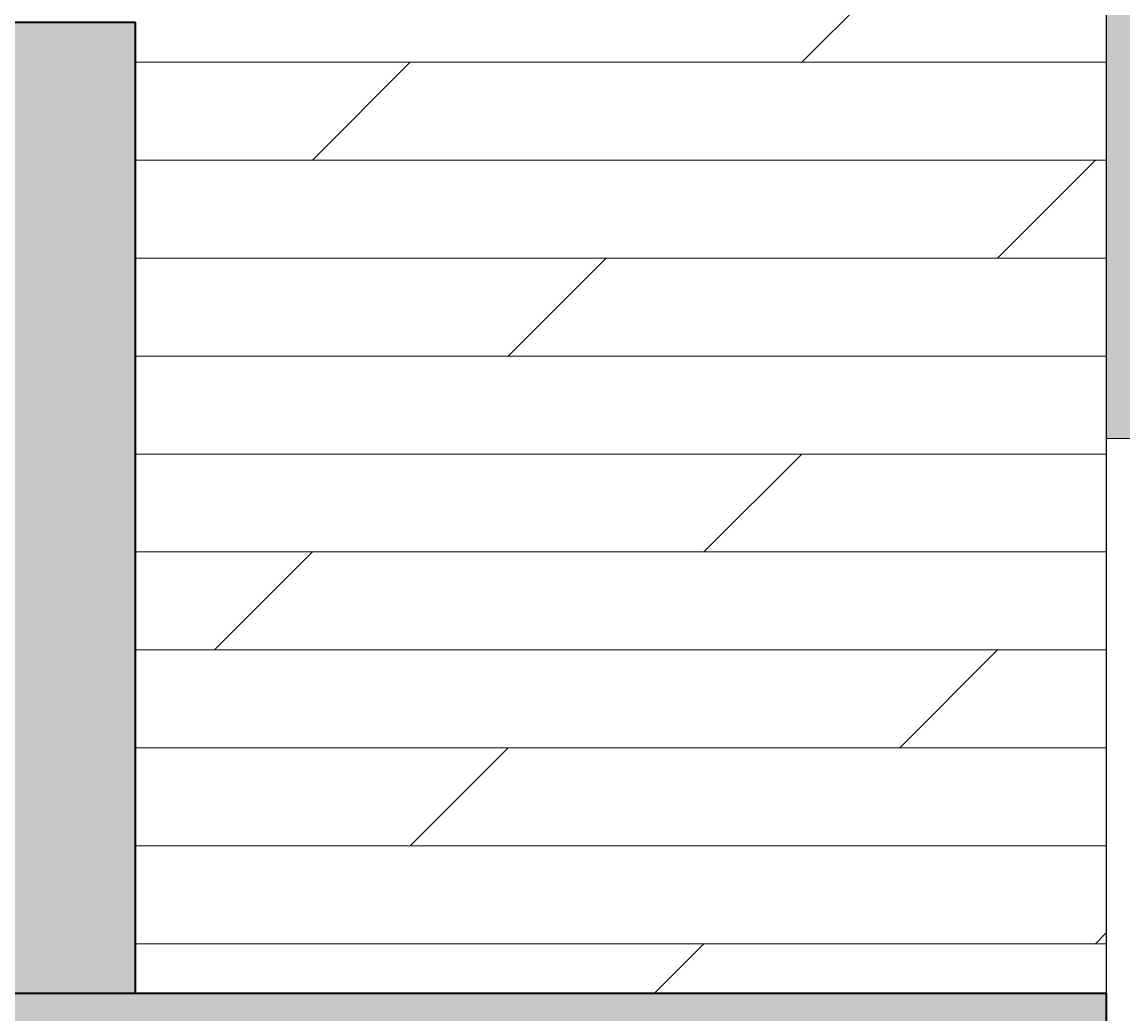
# Model space of a CAD drawing. Units: inches. Extents: x 84 to 1044, y -280 to 906.
# Tile 103 of 105: x 826 to 897, y 510 to 574. Entities that reach past the tile are written whole.
import ezdxf

# ---------------------------------------------------------------- set-up
doc = ezdxf.new("R2010")
doc.units = ezdxf.units.IN
for name, color, linetype, lineweight in [('A-ANNO-DIMS', 2, 'Continuous', 18), ('L-HRDS', 32, 'Continuous', 18), ('WALL', 250, 'Continuous', 35)]:
    doc.layers.add(name, color=color, linetype=linetype, lineweight=lineweight)
for name, color, linetype, lineweight, true_color in [('A-FLOR-PATT', 251, 'Continuous', 9, 0x705861), ('A-WALL-PATT', 251, 'Continuous', 9, 0x636466), ('L-PLNT-PATT', 9, 'Continuous', 9, 0xafd9aa)]:
    doc.layers.add(name, color=color, linetype=linetype, lineweight=lineweight, true_color=true_color)
doc.styles.get("Standard").update_dxf_attribs({"font": 'arial.ttf'})
doc.dimstyles.get("Standard").update_dxf_attribs({"dimtxt": 0.18, "dimasz": 0.18, "dimexe": 0.18, "dimexo": 0.0625, "dimgap": 0.09, "dimtad": 0, "dimtih": 1, "dimtoh": 1, "dimdec": 4, "dimzin": 0, "dimdsep": 46, "dimtxsty": 'Standard', "dimcen": 0.09, "dimadec": 0, "dimazin": 0, "dimtfac": 1, "dimtdec": 4, "dimtofl": 0, "dimtmove": 0, "dimatfit": 3, "dimfxl": 1, "dimtolj": 1, "dimtzin": 0, "dimarcsym": 0})

# ---------------------------------------------------------------- blocks, each defined once
blk = doc.blocks.new('*D62')
at = {"layer": 'A-ANNO-DIMS', "color": 0, "lineweight": -2, "transparency": 16777216}
for p, q in [((203.179, 709.183), (203.179, 905.9)), ((203.359, 905.72), (549.232, 905.72)), ((895.894, 905.72), (550.021, 905.72)), ((896.074, 400.183), (896.074, 905.9))]:
    blk.add_line(p, q, dxfattribs=at)
at = {"layer": 'A-ANNO-DIMS', "color": 0, "transparency": 16777216}
for points in [[(203.359, 905.75), (203.359, 905.69), (203.179, 905.72)], [(895.894, 905.75), (895.894, 905.69), (896.074, 905.72)]]:
    blk.add_solid(points, dxfattribs=at)
at = {"layer": 'Defpoints', "color": 0, "transparency": 16777216}
for p in [(896.074, 905.72), (203.179, 709.12), (896.074, 400.12)]:
    blk.add_point(p, dxfattribs=at)
at = {"layer": 'A-ANNO-DIMS', "color": 0, "transparency": 16777216, "insert": (549.627, 905.72), "char_height": 0.18, "attachment_point": 5}
blk.add_mtext('\\A1;692.9', dxfattribs=at)
blk = doc.blocks.new('*D63')
at = {"layer": 'A-ANNO-DIMS', "color": 0, "lineweight": -2, "transparency": 16777216}
for p, q in [((833.136, 709.12), (1043.768, 709.12)), ((1043.588, 708.94), (1043.588, 400.302)), ((1043.588, 91.3), (1043.588, 399.938)), ((896.136, 91.12), (1043.768, 91.12))]:
    blk.add_line(p, q, dxfattribs=at)
at = {"layer": 'A-ANNO-DIMS', "color": 0, "transparency": 16777216}
for points in [[(1043.558, 708.94), (1043.618, 708.94), (1043.588, 709.12)], [(1043.558, 91.3), (1043.618, 91.3), (1043.588, 91.12)]]:
    blk.add_solid(points, dxfattribs=at)
at = {"layer": 'Defpoints', "color": 0, "transparency": 16777216}
for p in [(833.074, 709.12), (1043.588, 709.12), (896.074, 91.12)]:
    blk.add_point(p, dxfattribs=at)
at = {"layer": 'A-ANNO-DIMS', "color": 0, "transparency": 16777216, "insert": (1043.588, 400.12), "char_height": 0.18, "attachment_point": 5}
blk.add_mtext('\\A1;618', dxfattribs=at)
blk = doc.blocks.new('*D65')
at = {"layer": 'A-ANNO-DIMS', "color": 0, "lineweight": -2, "transparency": 16777216}
for p, q in [((896.074, 400.183), (896.074, 905.9)), ((896.254, 905.72), (943.855, 905.72)), ((991.894, 905.72), (944.293, 905.72)), ((992.074, 856.183), (992.074, 905.9))]:
    blk.add_line(p, q, dxfattribs=at)
at = {"layer": 'A-ANNO-DIMS', "color": 0, "transparency": 16777216}
for points in [[(896.254, 905.75), (896.254, 905.69), (896.074, 905.72)], [(991.894, 905.75), (991.894, 905.69), (992.074, 905.72)]]:
    blk.add_solid(points, dxfattribs=at)
at = {"layer": 'Defpoints', "color": 0, "transparency": 16777216}
for p in [(896.074, 905.72), (992.074, 856.12), (896.074, 400.12)]:
    blk.add_point(p, dxfattribs=at)
at = {"layer": 'A-ANNO-DIMS', "color": 0, "transparency": 16777216, "insert": (944.074, 905.72), "char_height": 0.18, "attachment_point": 5}
blk.add_mtext('\\A1;96', dxfattribs=at)

msp = doc.modelspace()

# ---------------------------------------------------------------- hatches: boundary and pattern name
at = {"layer": 'A-FLOR-PATT', "transparency": 33554597}
h = msp.add_hatch(dxfattribs=at)
h.set_pattern_fill('DOLMIT', color=256)
h.paths.add_polyline_path([(896.074, 709.12), (833.074, 709.12), (833.074, 646.12), (833.074, 574.12), (833.074, 511.12), (896.074, 511.12)])
h.paths.add_polyline_path([(386.074, 769.12), (203.179, 769.12), (203.179, 709.12), (287.127, 709.12), (359.127, 709.12), (386.074, 709.12)])
at = {"layer": 'A-WALL-PATT', "transparency": 33554597}
h = msp.add_hatch(color=256, dxfattribs=at)
h.dxf.hatch_style = 1
h.paths.add_polyline_path([(671.074, 100.12), (647.074, 100.12), (647.074, 160.12), (641.074, 160.12), (620.824, 160.12), (620.824, 151.12), (638.074, 151.12), (638.074, 91.12), (671.074, 91.12)])
h.paths.add_polyline_path([(791.074, 100.12), (743.074, 100.12), (743.074, 91.12), (791.074, 91.12)])
h.paths.add_polyline_path([(896.074, 346.12), (887.074, 346.12), (887.074, 334.12), (870.955, 334.12), (833.074, 334.12), (804.574, 334.12), (804.574, 328.12), (887.074, 328.12), (887.074, 100.12), (863.074, 100.12), (863.074, 91.12), (896.074, 91.12)])
h.paths.add_polyline_path([(507.574, 154.729), (507.574, 160.12), (464.074, 160.12), (464.074, 247.12), (641.074, 247.12), (641.074, 208.12), (647.074, 208.12), (647.074, 328.12), (659.074, 328.12), (659.074, 334.12), (617.074, 334.12), (617.074, 328.12), (641.074, 328.12), (641.074, 256.12), (545.074, 256.12), (545.074, 328.12), (569.074, 328.12), (569.074, 334.12), (518.074, 334.12), (518.074, 325.12), (536.074, 325.12), (536.074, 256.12), (464.074, 256.12), (464.074, 325.12), (482.074, 325.12), (482.074, 334.12), (455.074, 334.12), (455.074, 160.12), (413.127, 160.12), (413.127, 151.12), (455.074, 151.12), (455.074, 91.12), (464.074, 91.12), (464.074, 151.12), (507.574, 151.12)])
h.paths.add_polyline_path([(572.824, 160.12), (555.574, 160.12), (555.574, 151.12), (572.824, 151.12)], flags=17)
h.paths.add_polyline_path([(341.127, 160.12), (299.179, 160.12), (299.179, 211.12), (294.179, 211.12), (290.179, 211.12), (290.179, 151.12), (341.127, 151.12)])
h.paths.add_polyline_path([(299.179, 256.12), (212.179, 256.12), (212.179, 274.12), (203.179, 274.12), (203.179, 247.12), (299.179, 247.12)])
h.paths.add_polyline_path([(212.179, 514.12), (398.074, 514.12), (398.074, 519.12), (398.074, 520.12), (212.179, 520.12), (212.179, 574.12), (203.179, 574.12), (203.179, 310.12), (212.179, 310.12), (212.179, 328.12), (290.179, 328.12), (290.179, 292.12), (299.179, 292.12), (299.179, 328.12), (332.179, 328.12), (332.179, 334.12), (212.179, 334.12)])
h.paths.add_polyline_path([(287.127, 709.12), (203.179, 709.12), (203.179, 646.12), (212.179, 646.12), (212.179, 700.12), (287.127, 700.12)])
h.paths.add_polyline_path([(470.074, 709.12), (359.127, 709.12), (359.127, 700.12), (434.074, 700.12), (434.074, 574.12), (440.074, 574.12), (440.074, 622.12), (464.074, 622.12), (464.074, 628.12), (440.074, 628.12), (440.074, 700.12), (470.074, 700.12)])
h.paths.add_polyline_path([(572.074, 709.12), (506.074, 709.12), (506.074, 700.12), (536.074, 700.12), (536.074, 628.12), (494.074, 628.12), (494.074, 622.12), (536.074, 622.12), (536.074, 520.12), (440.074, 520.12), (440.074, 544.12), (434.074, 544.12), (434.074, 514.12), (644.074, 514.12), (644.074, 519.12), (644.074, 544.12), (638.074, 544.12), (638.074, 520.12), (542.074, 520.12), (542.074, 622.12), (584.074, 622.12), (584.074, 628.12), (542.074, 628.12), (542.074, 700.12), (572.074, 700.12)])
h.paths.add_polyline_path([(698.074, 709.12), (608.074, 709.12), (608.074, 700.12), (638.074, 700.12), (638.074, 628.12), (614.074, 628.12), (614.074, 622.12), (638.074, 622.12), (638.074, 574.12), (644.074, 574.12), (644.074, 700.12), (698.074, 700.12)])
h.paths.add_polyline_path([(833.074, 709.12), (770.074, 709.12), (770.074, 700.12), (824.074, 700.12), (824.074, 646.12), (833.074, 646.12)])
h.paths.add_polyline_path([(833.074, 574.12), (824.074, 574.12), (824.074, 520.12), (791.244, 520.12), (712.904, 520.12), (680.074, 520.12), (680.074, 514.12), (695.074, 514.12), (695.074, 491.62), (704.074, 491.62), (704.074, 511.12), (833.074, 511.12)])
h.paths.add_polyline_path([(704.074, 419.62), (695.074, 419.62), (695.074, 370.12), (704.074, 370.12)])
h.paths.add_polyline_path([(896.074, 400.12), (833.074, 400.12), (833.074, 364.12), (839.074, 364.12), (839.074, 394.12), (887.074, 394.12), (887.074, 382.12), (896.074, 382.12)])
h.paths.add_polyline_path([(732.574, 334.12), (695.074, 334.12), (695.074, 328.12), (732.574, 328.12)])
at = {"layer": 'L-PLNT-PATT', "transparency": 33554597}
h = msp.add_hatch(color=256, dxfattribs=at)
h.dxf.hatch_style = 1
h.paths.add_polyline_path([(434.074, 769.12), (386.074, 769.12), (386.074, 709.12), (434.074, 709.12)])
h.paths.add_polyline_path([(896.074, 847.12), (434.074, 847.12), (434.074, 769.12), (434.074, 709.12), (470.074, 709.12), (506.074, 709.12), (572.074, 709.12), (608.074, 709.12), (698.074, 709.12), (770.074, 709.12), (833.074, 709.12), (896.074, 709.12)])
h.paths.add_polyline_path([(983.074, 847.12), (896.074, 847.12), (896.074, 709.12), (896.074, 547.12), (932.074, 547.12), (983.074, 547.12)])
h.paths.add_polyline_path([(983.074, 547.12), (932.074, 547.12), (932.074, 265.12), (983.074, 265.12)])
h.paths.add_polyline_path([(203.179, 646.12), (203.179, 709.12), (203.179, 745.12), (143.179, 745.12), (143.179, 271.12), (203.179, 271.12), (203.179, 274.12), (203.179, 310.12), (203.179, 574.12)])
h = msp.add_hatch(color=256, dxfattribs=at)
h.dxf.hatch_style = 1
h.paths.add_polyline_path([(896.074, 511.12), (704.074, 511.12), (704.074, 491.62), (704.074, 419.62), (704.074, 400.12), (833.074, 400.12), (896.074, 400.12)])

# ---------------------------------------------------------------- linework, layer by layer
at = {"layer": 'L-HRDS'}
for p, q in [((896.074, 511.12), (896.074, 709.12)), ((932.074, 547.12), (896.074, 547.12))]:
    msp.add_line(p, q, dxfattribs=at)
at = {"layer": 'WALL'}
for p, q in [((824.074, 574.12), (833.074, 574.12)), ((833.074, 511.12), (833.074, 574.12)), ((896.074, 511.12), (704.074, 511.12)), ((896.074, 400.12), (896.074, 511.12))]:
    msp.add_line(p, q, dxfattribs=at)

# ---------------------------------------------------------------- dimensions: what is measured, and where the dimension line sits
at = {"layer": 'A-ANNO-DIMS'}
for p1, override, picture, middle in [((203.179, 709.12), {"dimdec": 1, "dimlfac": 1, "dimrnd": 0, "dimzin": 0, "dimdsep": 46, "dimlunit": 2}, '*D62', (549.627, 905.72)), ((992.074, 856.12), {"dimdec": 0, "dimlfac": 1, "dimrnd": 0, "dimzin": 0, "dimdsep": 46, "dimlunit": 2}, '*D65', (944.074, 905.72))]:
    dim = msp.add_linear_dim(base=(896.074, 905.72), p1=p1, p2=(896.074, 400.12), dimstyle='Standard', override=override, dxfattribs=at)
    dim.commit()
    dim.dimension.update_dxf_attribs({"geometry": picture, "text_midpoint": middle})
dim = msp.add_linear_dim(base=(1043.588, 709.12), p1=(896.074, 91.12), p2=(833.074, 709.12), angle=90, dimstyle='Standard', override={"dimdec": 0, "dimlfac": 1, "dimrnd": 0, "dimzin": 0, "dimdsep": 46, "dimlunit": 2}, dxfattribs=at)
dim.commit()
dim.dimension.update_dxf_attribs({"geometry": '*D63', "text_midpoint": (1043.588, 400.12)})

doc.saveas('drawing.dxf')
